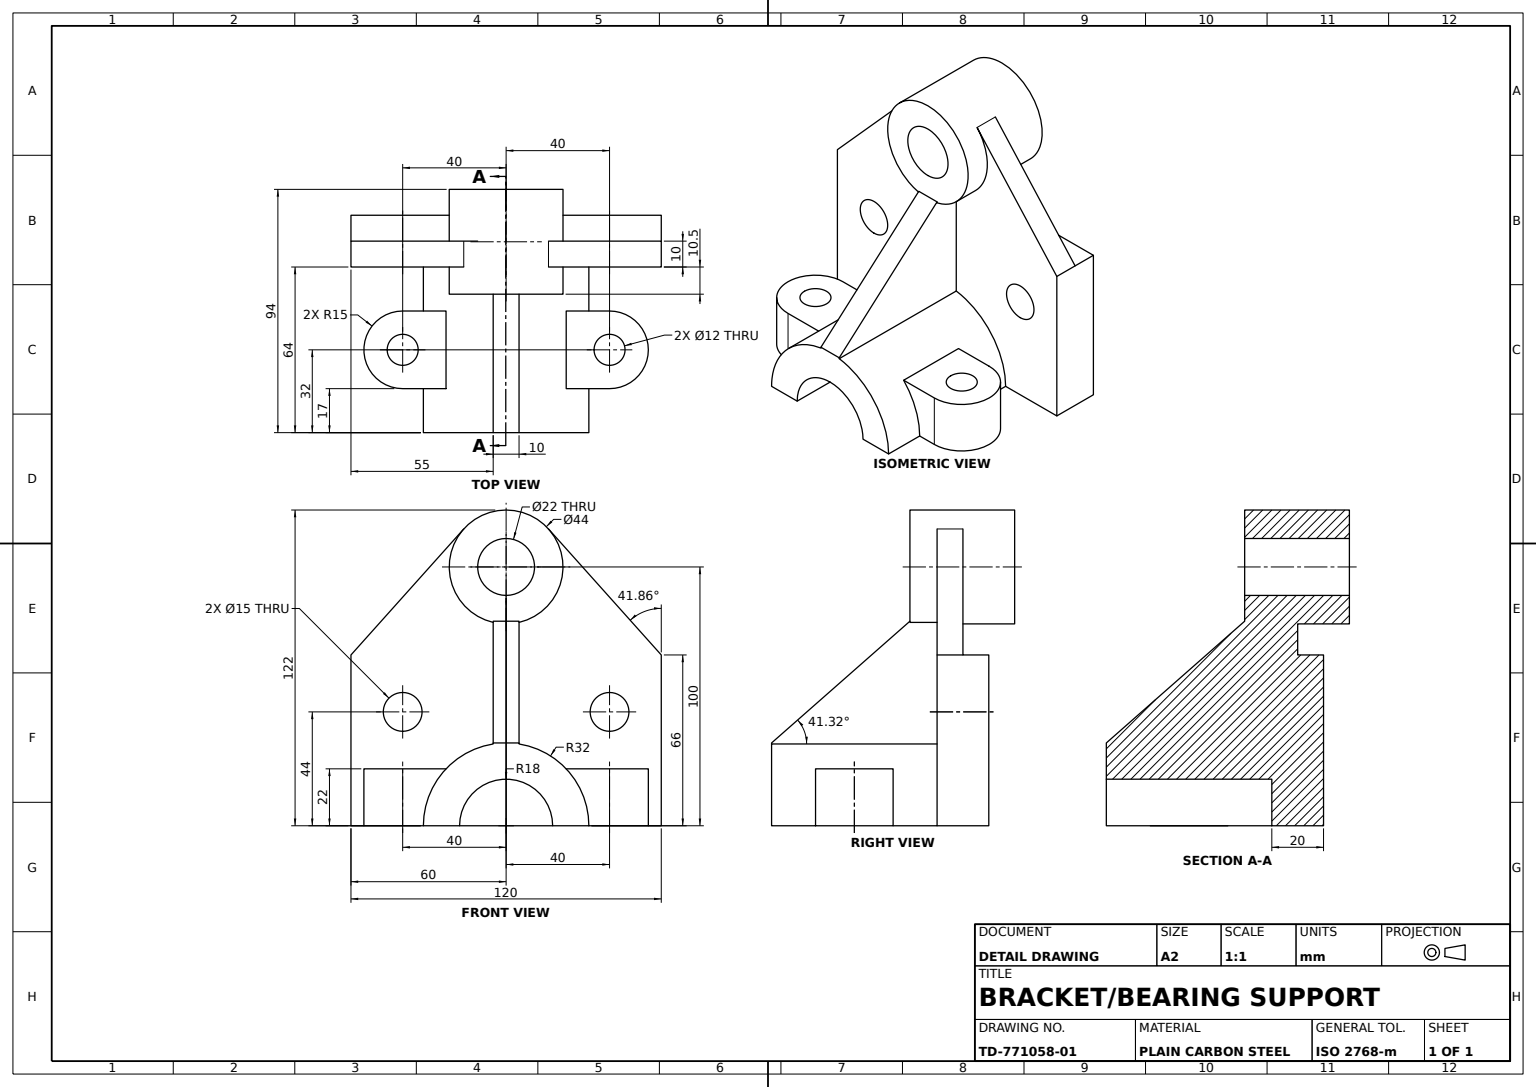
SolidWorks part; units mm, degrees
material "Plain Carbon Steel"
ref_plane "Front Plane" through (0, 0, 0) normal (0, 0, 1) x (1, 0, 0)
ref_plane "Top Plane" through (0, 0, 0) normal (0, 1, 0) x (1, 0, 0)
ref_plane "Right Plane" through (0, 0, 0) normal (1, 0, 0) x (0, 0, -1)
sketch "Base Plate Sketch" plane through (0, 0, 0) normal (0, 0, 1) x (1, 0, 0)
  line L1 (-10, 33) -> (10, 33)
  line L2 (-10, 33) -> (-10, -33)
  line L3 (-10, -33) -> (10, -33)
  line L4 (10, 33) -> (10, -33)
  line L5 (-10, 33) -> (10, -33) construction
  line L6 (-10, -33) -> (10, 33) construction
  point P0 (0, 0)
  dimension "D1" = 66
  dimension "D2" = 20
extrude "Base Plate" add sketch "Base Plate Sketch" along normal blind 120
sketch "Upright Web Sketch" plane through (10, 0, 0) normal (1, 0, 0) x (0, 0, -1)
  line L0 (-120, -33) -> (0, -33) construction
  line L1 (0, -33) -> (0, 33) construction
  line L2 (-120, 33) -> (-76.3856, 81.6804)
  line L3 (0, 33) -> (-43.6144, 81.6804)
  line L4 (-120, 33) -> (0, 33)
  circle A0 centre (-60, 67) radius 11
  circle A1 centre (-60, 67) radius 22
  line M2 (0, 33) -> (-120, 33)
  dimension "D1" = 22
  dimension "D2" = 44
  dimension "D3" = 100
  dimension "D4" = 60
extrude "Upright Web" add sketch "Upright Web Sketch" against normal blind 10 contours A1 L2 L3 M2 | A1 A0
sketch "Trunnion Boss Front Sketch" plane through (0, 0, 0) normal (-1, 0, 0) x (0, 0, 1)
  circle A0 centre (60, 67) radius 11
  circle A1 centre (60, 67) radius 22
  dimension "D1" = 44
  dimension "D2" = 22
extrude "Trunnion Boss Front" add sketch "Trunnion Boss Front Sketch" along normal blind 20
sketch "Trunnion Boss Rear Sketch" plane through (10, 0, 0) normal (1, 0, 0) x (0, 0, -1)
  circle A0 centre (-60, 67) radius 11
  circle A1 centre (-60, 67) radius 22
  dimension "D1" = 44
  dimension "D2" = 22
extrude "Trunnion Boss Rear" add sketch "Trunnion Boss Rear Sketch" along normal blind 10
sketch "Bracket Holes Sketch" plane through (10, 0, 0) normal (1, 0, 0) x (0, 0, -1)
  line L0 (-60, 45) -> (-60, 67)
  line L1 (-120, -33) -> (0, -33) construction
  circle A0 centre (-100, 11) radius 7.5
  circle A1 centre (-20, 11) radius 7.5
  arc A2 (-76.3856, 81.6804) -> (-43.6144, 81.6804) centre (-60, 67) ccw construction
  dimension "D1" = 15
  dimension "D2" = 15
  dimension "D3" = 40
  dimension "D4" = 40
  dimension "D5" = 44
  dimension "D6" = 44
extrude "Bracket Holes" cut sketch "Bracket Holes Sketch" against normal blind 30 contours A0 | A1
sketch "Semi-Circular Base Sketch" plane through (10, 0, 0) normal (1, 0, 0) x (0, 0, -1)
  line L0 (-120, -33) -> (0, -33) construction
  line L1 (-92, -33) -> (-78, -33)
  line L2 (-42, -33) -> (-28, -33)
  arc A0 (-28, -33) -> (-92, -33) centre (-60, -33) ccw
  arc A1 (-42, -33) -> (-78, -33) centre (-60, -33) ccw
  dimension "D1" = 64
  dimension "D2" = 36
extrude "Semi-Circular Base" add sketch "Semi-Circular Base Sketch" along normal blind 64
ref_plane "Gusset Plane" through (0, 0, 60) normal (0, 0, 1) x (1, 0, 0)
sketch "Gusset 1 Sketch" plane through (0, 0, 60) normal (0, 0, 1) x (1, 0, 0)
  line L4 (10, -5) -> (10, 46.4788)
  line L6 (10, -33) -> (10, 33) construction
  line L7 (10, -5) -> (74, -5)
  line L8 (74, -33) -> (74, -1) construction
  line L9 (74, -5) -> (74, -1)
  line L10 (10, 45) -> (10, 81.6804) construction
  line L11 (10, 46.4788) -> (20, 46.4788)
  line L12 (20, 45) -> (20, 89) construction
  line L13 (20, 46.4788) -> (74, -1)
  dimension "D1" = 51.4788
  dimension "D2" = 47.4788
extrude "Gusset 1" add sketch "Gusset 1 Sketch" along normal mid plane 10 separate body
sketch "Gusset 2 Sketch" plane through (74, 0, 0) normal (1, 0, 0) x (0, 0, -1)
  line L0 (-92, -33) -> (-78, -33)
  line L1 (-42, -33) -> (-28, -33)
  arc A0 (-92, -33) -> (-28, -33) centre (-60, -33) cw
  arc A1 (-28, -33) -> (-92, -33) centre (-60, -33) ccw construction
  arc A2 (-28, -33) -> (-92, -33) centre (-60, -33) ccw construction
  arc A3 (-78, -33) -> (-42, -33) centre (-60, -33) cw
  dimension "D1" = 32
  dimension "D2" = 18
extrude "Gusset 2" add sketch "Gusset 2 Sketch" against normal up to surface (64 mm away) up to face at (10, 18.5, 20)
sketch "Trunnion Face Pad Sketch" plane through (20, 0, 0) normal (1, 0, 0) x (0, 0, -1)
  circle A0 centre (-60, 67) radius 11
  circle A1 centre (-60, 67) radius 22
  dimension "D1" = 44
  dimension "D2" = 22
extrude "Trunnion Face Pad 0.5mm" add sketch "Trunnion Face Pad Sketch" along normal blind 0.5
sketch "Base Mounting Lugs Sketch" plane through (0, -33, 0) normal (0, -1, 0) x (1, 0, 0)
  line L0 (10, 42) -> (10, 78) construction
  line L1 (10, 120) -> (10, 92) construction
  line L2 (27, 100) -> (27, 83)
  line L4 (57, 85) -> (57, 100)
  line L6 (10, 28) -> (10, 0) construction
  line L7 (27, 20) -> (27, 38)
  line L9 (57, 35) -> (57, 20)
  line L10 (27, 38) -> (57, 38)
  line L11 (57, 38) -> (57, 35)
  line L12 (27, 83) -> (57, 83)
  line L13 (57, 83) -> (57, 85)
  arc A0 (57, 100) -> (27, 100) centre (42, 100) ccw
  circle A1 centre (42, 100) radius 6
  circle A2 centre (42, 20) radius 6
  arc A3 (27, 20) -> (57, 20) centre (42, 20) ccw
  point P5 (10, 60)
  dimension "D1" = 30
  dimension "D2" = 12
  dimension "D5" = 30
  dimension "D6" = 12
  dimension "D3" = 40
  dimension "D4" = 32
  dimension "D7" = 40
  dimension "D8" = 32
  dimension "D9" = 15
  dimension "D10" = 18
  dimension "D11" = 17
  dimension "D12" = 30
  dimension "D13" = 2
  dimension "D14" = 3
extrude "Base Mounting Lugs" add sketch "Base Mounting Lugs Sketch" against normal blind 22
